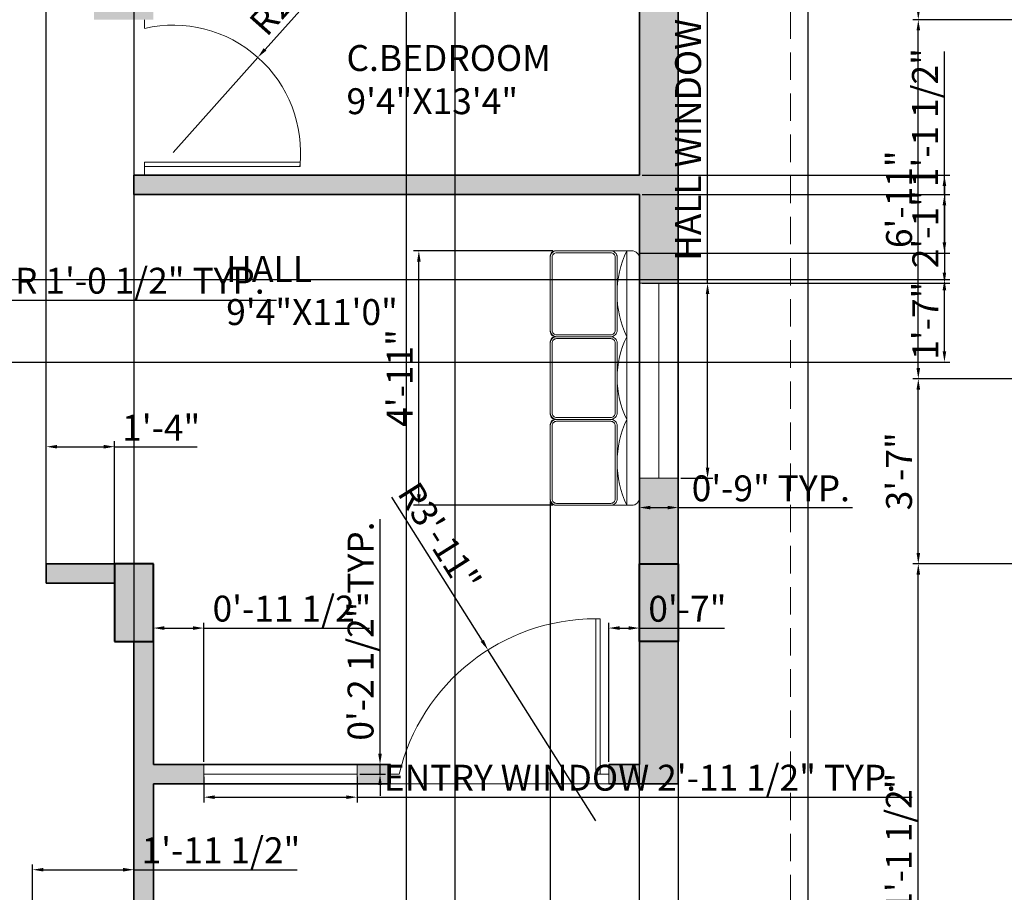
# Model space of a CAD drawing. Units: inches. Extents: x 2656 to 9931, y 1941 to 3068.
# Tile 3 of 46: x 2846 to 3074, y 2224 to 2426. Entities that reach past the tile are written whole.
import ezdxf

# ---------------------------------------------------------------- set-up
doc = ezdxf.new("R2010")
doc.units = ezdxf.units.IN
doc.linetypes.add('DASHED2', pattern=[9.525, 6.35, -3.175])
for name, color, linetype, lineweight in [('A-ANNO-DIMS', 2, 'Continuous', 18), ('A-AREA-IDEN', 7, 'Continuous', 18), ('A-COLS', 7, 'Continuous', 40), ('A-COLS-PATT', 146, 'Continuous', 13), ('A-DOOR', 3, 'Continuous', 18), ('A-FLOR-OVHD', 252, 'DASHED2', 13), ('A-FURN', 8, 'Continuous', 13), ('A-GLAZ', 4, 'Continuous', 18), ('A-WALL', 7, 'Continuous', 35), ('A-WALL-PATT', 251, 'Continuous', 13), ('C-PROP', 7, 'Continuous', 25)]:
    doc.layers.add(name, color=color, linetype=linetype, lineweight=lineweight)
doc.styles.get("Standard").update_dxf_attribs({"font": 'arial.ttf'})
doc.dimstyles.new('ISO-25', dxfattribs={"dimtxt": 6, "dimasz": 2.5, "dimexe": 1.25, "dimexo": 0.625, "dimtad": 1, "dimdec": 0, "dimlunit": 3, "dimtxsty": 'Standard', "dimcen": 2.5, "dimadec": 0, "dimazin": 0, "dimtfac": 1, "dimtdec": 0, "dimtmove": 0, "dimatfit": 3, "dimfxl": 1, "dimarcsym": 0})

# ---------------------------------------------------------------- blocks, each defined once
blk = doc.blocks.new('DOOR-BEDROOM-HALL')
for p, q in [((-0.04, 0), (-0.04, 36)), ((2.43, 36), (2.43, 34)), ((38.43, 3), (2.43, 3)), ((2.43, 3), (2.43, 2)), ((38.43, 2), (38.43, 3)), ((2.43, 0), (2.43, 2)), ((2.43, 2), (38.43, 2))]:
    blk.add_line(p, q)
blk.add_arc((9.01, 5.24), 29.5, 353.6889, 102.8962)
blk = doc.blocks.new('DOOR-ENTRY')
for p, q in [((48.56, 38.25), (47.56, 38.25)), ((47.56, 38.25), (47.56, 2.25)), ((48.56, 2.25), (48.56, 38.25)), ((0.04, 2.25), (2.04, 2.25)), ((0.04, 0), (50.56, 0)), ((47.56, 2.25), (48.56, 2.25)), ((50.56, 2.25), (48.56, 2.25))]:
    blk.add_line(p, q)
blk.add_arc((47.56, -8.52), 46.77, 90, 166.6828)
blk = doc.blocks.new('WIN-HALL')
for p, q in [((8.96, 45.14), (4.46, 45.14)), ((4.46, 45.14), (4.46, -0.02)), ((4.46, -0.02), (-0.04, -0.02))]:
    blk.add_line(p, q)
blk = doc.blocks.new('WIN-ENTRY')
for p, q in [((35.5, -0.05), (35.5, 2.2)), ((0.02, -0.05), (35.5, -0.05))]:
    blk.add_line(p, q)
blk = doc.blocks.new('*D47')
at = {"layer": 'A-ANNO-DIMS', "color": 0, "lineweight": -2, "transparency": 16777216}
for p, q in [((3004.93, 2365.04), (3004.93, 2467.44)), ((2998.78, 2365.04), (3006.18, 2365.04)), ((3004.93, 2322.38), (3004.93, 2362.54)), ((2998.78, 2319.88), (3006.18, 2319.88))]:
    blk.add_line(p, q, dxfattribs=at)
at = {"layer": 'A-ANNO-DIMS', "color": 0, "transparency": 16777216}
for points in [[(3004.51, 2362.54), (3005.35, 2362.54), (3004.93, 2365.04)], [(3004.51, 2322.38), (3005.35, 2322.38), (3004.93, 2319.88)]]:
    blk.add_solid(points, dxfattribs=at)
at = {"layer": 'Defpoints', "color": 0, "transparency": 16777216}
for p in [(2998.16, 2365.04), (3004.93, 2365.04), (2998.16, 2319.88)]:
    blk.add_point(p, dxfattribs=at)
at = {"layer": 'A-ANNO-DIMS', "color": 0, "transparency": 16777216, "insert": (3001.2, 2417.49), "char_height": 6, "attachment_point": 5, "rotation": 90}
blk.add_mtext('HALL WINDOW 3\'-9" TYP.', dxfattribs=at)
blk = doc.blocks.new('*D48')
at = {"layer": 'A-ANNO-DIMS', "color": 0, "lineweight": -2, "transparency": 16777216}
for p, q in [((2989.16, 2319.25), (2989.16, 2311.86)), ((2998.16, 2319.25), (2998.16, 2311.86)), ((2991.66, 2313.11), (2995.66, 2313.11)), ((2998.16, 2313.11), (3038.48, 2313.11))]:
    blk.add_line(p, q, dxfattribs=at)
at = {"layer": 'A-ANNO-DIMS', "color": 0, "transparency": 16777216}
for points in [[(2991.66, 2313.52), (2991.66, 2312.69), (2989.16, 2313.11)], [(2995.66, 2313.52), (2995.66, 2312.69), (2998.16, 2313.11)]]:
    blk.add_solid(points, dxfattribs=at)
at = {"layer": 'Defpoints', "color": 0, "transparency": 16777216}
for p in [(2989.16, 2319.88), (2998.16, 2319.88), (2998.16, 2313.11)]:
    blk.add_point(p, dxfattribs=at)
at = {"layer": 'A-ANNO-DIMS', "color": 0, "transparency": 16777216, "insert": (3019.57, 2316.79), "char_height": 6, "attachment_point": 5}
blk.add_mtext('0\'-9" TYP.', dxfattribs=at)
blk = doc.blocks.new('*D49')
at = {"layer": 'A-ANNO-DIMS', "color": 0, "lineweight": -2, "transparency": 16777216}
for p, q in [((2888.32, 2250.73), (2888.32, 2244.78)), ((2923.8, 2250.73), (2923.8, 2244.78)), ((2890.82, 2246.03), (2921.3, 2246.03)), ((2923.8, 2246.03), (3052.29, 2246.03))]:
    blk.add_line(p, q, dxfattribs=at)
at = {"layer": 'A-ANNO-DIMS', "color": 0, "transparency": 16777216}
for points in [[(2890.82, 2246.45), (2890.82, 2245.61), (2888.32, 2246.03)], [(2921.3, 2246.45), (2921.3, 2245.61), (2923.8, 2246.03)]]:
    blk.add_solid(points, dxfattribs=at)
at = {"layer": 'Defpoints', "color": 0, "transparency": 16777216}
for p in [(2888.32, 2251.35), (2923.8, 2251.35), (2923.8, 2246.03)]:
    blk.add_point(p, dxfattribs=at)
at = {"layer": 'A-ANNO-DIMS', "color": 0, "transparency": 16777216, "insert": (2989.29, 2249.76), "char_height": 6, "attachment_point": 5}
blk.add_mtext('ENTRY WINDOW 2\'-11 1/2" TYP.', dxfattribs=at)
blk = doc.blocks.new('*D50')
at = {"layer": 'A-ANNO-DIMS', "color": 0, "lineweight": -2, "transparency": 16777216}
for p, q in [((2929.12, 2256.1), (2929.12, 2310.4)), ((2924.42, 2253.6), (2930.37, 2253.6)), ((2929.12, 2251.35), (2929.12, 2253.6)), ((2924.42, 2251.35), (2930.37, 2251.35)), ((2929.12, 2248.85), (2929.12, 2246.35))]:
    blk.add_line(p, q, dxfattribs=at)
at = {"layer": 'A-ANNO-DIMS', "color": 0, "transparency": 16777216}
for points in [[(2928.7, 2256.1), (2929.53, 2256.1), (2929.12, 2253.6)], [(2928.7, 2248.85), (2929.53, 2248.85), (2929.12, 2251.35)]]:
    blk.add_solid(points, dxfattribs=at)
at = {"layer": 'Defpoints', "color": 0, "transparency": 16777216}
for p in [(2923.8, 2253.6), (2929.12, 2253.6), (2923.8, 2251.35)]:
    blk.add_point(p, dxfattribs=at)
at = {"layer": 'A-ANNO-DIMS', "color": 0, "transparency": 16777216, "insert": (2925.39, 2284.5), "char_height": 6, "attachment_point": 5, "rotation": 90}
blk.add_mtext('0\'-2 1/2" TYP.', dxfattribs=at)
blk = doc.blocks.new('*D61')
at = {"layer": 'A-ANNO-DIMS', "color": 0, "lineweight": -2, "transparency": 16777216}
for p, q in [((2778.76, 2362.36), (2778.76, 2359.89)), ((2781.26, 2361.14), (2788.58, 2361.14)), ((2791.08, 2362.36), (2791.08, 2359.89)), ((2791.08, 2361.14), (2905.16, 2361.14))]:
    blk.add_line(p, q, dxfattribs=at)
at = {"layer": 'A-ANNO-DIMS', "color": 0, "transparency": 16777216}
for points in [[(2781.26, 2361.55), (2781.26, 2360.72), (2778.76, 2361.14)], [(2788.58, 2361.55), (2788.58, 2360.72), (2791.08, 2361.14)]]:
    blk.add_solid(points, dxfattribs=at)
at = {"layer": 'Defpoints', "color": 0, "transparency": 16777216}
for p in [(2778.76, 2362.98), (2791.08, 2362.98), (2791.08, 2361.14)]:
    blk.add_point(p, dxfattribs=at)
at = {"layer": 'A-ANNO-DIMS', "color": 0, "transparency": 16777216, "insert": (2849.37, 2364.86), "char_height": 6, "attachment_point": 5}
blk.add_mtext('DINING CHAIR 1\'-0 1/2" TYP.', dxfattribs=at)
blk = doc.blocks.new('*D69')
at = {"layer": 'A-ANNO-DIMS', "color": 0, "lineweight": -2, "transparency": 16777216}
for p, q in [((3144.42, 2300.1), (3052.46, 2300.1)), ((3053.71, 2169.1), (3053.71, 2297.6)), ((3144.42, 2166.6), (3052.46, 2166.6))]:
    blk.add_line(p, q, dxfattribs=at)
at = {"layer": 'A-ANNO-DIMS', "color": 0, "transparency": 16777216}
for points in [[(3053.3, 2297.6), (3054.13, 2297.6), (3053.71, 2300.1)], [(3053.3, 2169.1), (3054.13, 2169.1), (3053.71, 2166.6)]]:
    blk.add_solid(points, dxfattribs=at)
at = {"layer": 'Defpoints', "color": 0, "transparency": 16777216}
for p in [(3053.71, 2300.1), (3145.05, 2300.1), (3145.05, 2166.6)]:
    blk.add_point(p, dxfattribs=at)
at = {"layer": 'A-ANNO-DIMS', "color": 0, "transparency": 16777216, "insert": (3049.99, 2233.35), "char_height": 6, "attachment_point": 5, "rotation": 90}
blk.add_mtext('11\'-1 1/2"', dxfattribs=at)
blk = doc.blocks.new('*D70')
at = {"layer": 'A-ANNO-DIMS', "color": 0, "lineweight": -2, "transparency": 16777216}
for p, q in [((3088.25, 2342.93), (3052.46, 2342.93)), ((3053.71, 2302.6), (3053.71, 2340.43)), ((3144.42, 2300.1), (3052.46, 2300.1))]:
    blk.add_line(p, q, dxfattribs=at)
at = {"layer": 'A-ANNO-DIMS', "color": 0, "transparency": 16777216}
for points in [[(3053.3, 2340.43), (3054.13, 2340.43), (3053.71, 2342.93)], [(3053.3, 2302.6), (3054.13, 2302.6), (3053.71, 2300.1)]]:
    blk.add_solid(points, dxfattribs=at)
at = {"layer": 'Defpoints', "color": 0, "transparency": 16777216}
for p in [(3053.71, 2342.93), (3088.87, 2342.93), (3145.05, 2300.1)]:
    blk.add_point(p, dxfattribs=at)
at = {"layer": 'A-ANNO-DIMS', "color": 0, "transparency": 16777216, "insert": (3050.02, 2321.51), "char_height": 6, "attachment_point": 5, "rotation": 90}
blk.add_mtext('3\'-7"', dxfattribs=at)
blk = doc.blocks.new('*D71')
at = {"layer": 'A-ANNO-DIMS', "color": 0, "lineweight": -2, "transparency": 16777216}
for p, q in [((3144.42, 2426.1), (3052.46, 2426.1)), ((3053.71, 2345.43), (3053.71, 2423.6)), ((3088.25, 2342.93), (3052.46, 2342.93))]:
    blk.add_line(p, q, dxfattribs=at)
at = {"layer": 'A-ANNO-DIMS', "color": 0, "transparency": 16777216}
for points in [[(3053.3, 2423.6), (3054.13, 2423.6), (3053.71, 2426.1)], [(3053.3, 2345.43), (3054.13, 2345.43), (3053.71, 2342.93)]]:
    blk.add_solid(points, dxfattribs=at)
at = {"layer": 'Defpoints', "color": 0, "transparency": 16777216}
for p in [(3053.71, 2426.1), (3145.05, 2426.1), (3088.87, 2342.93)]:
    blk.add_point(p, dxfattribs=at)
at = {"layer": 'A-ANNO-DIMS', "color": 0, "transparency": 16777216, "insert": (3050.03, 2384.51), "char_height": 6, "attachment_point": 5, "rotation": 90}
blk.add_mtext('6\'-11"', dxfattribs=at)
blk = doc.blocks.new('*D72')
at = {"layer": 'A-ANNO-DIMS', "color": 0, "lineweight": -2, "transparency": 16777216}
for p, q in [((3144.42, 2484.03), (3052.46, 2484.03)), ((3053.71, 2428.6), (3053.71, 2481.53)), ((3144.42, 2426.1), (3052.46, 2426.1))]:
    blk.add_line(p, q, dxfattribs=at)
at = {"layer": 'A-ANNO-DIMS', "color": 0, "transparency": 16777216}
for points in [[(3053.3, 2481.53), (3054.13, 2481.53), (3053.71, 2484.03)], [(3053.3, 2428.6), (3054.13, 2428.6), (3053.71, 2426.1)]]:
    blk.add_solid(points, dxfattribs=at)
at = {"layer": 'Defpoints', "color": 0, "transparency": 16777216}
for p in [(3053.71, 2484.03), (3145.05, 2484.03), (3145.05, 2426.1)]:
    blk.add_point(p, dxfattribs=at)
at = {"layer": 'A-ANNO-DIMS', "color": 0, "transparency": 16777216, "insert": (3050.03, 2455.07), "char_height": 6, "attachment_point": 5, "rotation": 90}
blk.add_mtext('4\'-10"', dxfattribs=at)
blk = doc.blocks.new('*D74')
at = {"layer": 'A-ANNO-DIMS', "color": 0, "lineweight": -2, "transparency": 16777216}
for p, q in [((2989.78, 2390.1), (3061.01, 2390.1)), ((3059.76, 2387.6), (3059.76, 2367.54)), ((2989.78, 2365.04), (3061.01, 2365.04))]:
    blk.add_line(p, q, dxfattribs=at)
at = {"layer": 'A-ANNO-DIMS', "color": 0, "transparency": 16777216}
for points in [[(3059.34, 2387.6), (3060.17, 2387.6), (3059.76, 2390.1)], [(3059.34, 2367.54), (3060.17, 2367.54), (3059.76, 2365.04)]]:
    blk.add_solid(points, dxfattribs=at)
at = {"layer": 'Defpoints', "color": 0, "transparency": 16777216}
for p in [(2989.16, 2390.1), (2989.16, 2365.04), (3059.76, 2365.04)]:
    blk.add_point(p, dxfattribs=at)
at = {"layer": 'A-ANNO-DIMS', "color": 0, "transparency": 16777216, "insert": (3056.12, 2377.57), "char_height": 6, "attachment_point": 5, "rotation": 90}
blk.add_mtext('2\'-1"', dxfattribs=at)
blk = doc.blocks.new('*D101')
at = {"layer": 'A-ANNO-DIMS', "color": 0, "lineweight": -2, "transparency": 16777216}
for p, q in [((2935.16, 2553.98), (2935.16, 2009.27)), ((2946.47, 2553.98), (2946.47, 2009.27)), ((2937.66, 2010.52), (2943.97, 2010.52)), ((2946.47, 2010.52), (2984.81, 2010.52))]:
    blk.add_line(p, q, dxfattribs=at)
at = {"layer": 'A-ANNO-DIMS', "color": 0, "transparency": 16777216}
for points in [[(2937.66, 2010.94), (2937.66, 2010.11), (2935.16, 2010.52)], [(2943.97, 2010.94), (2943.97, 2010.11), (2946.47, 2010.52)]]:
    blk.add_solid(points, dxfattribs=at)
at = {"layer": 'Defpoints', "color": 0, "transparency": 16777216}
for p in [(2935.16, 2554.6), (2946.47, 2554.6), (2946.47, 2010.52)]:
    blk.add_point(p, dxfattribs=at)
at = {"layer": 'A-ANNO-DIMS', "color": 0, "transparency": 16777216, "insert": (2966.89, 2014.25), "char_height": 6, "attachment_point": 5}
blk.add_mtext('0\'-11 1/2"', dxfattribs=at)
blk = doc.blocks.new('*D102')
at = {"layer": 'A-ANNO-DIMS', "color": 0, "lineweight": -2, "transparency": 16777216}
for p, q in [((2998.16, 2604.98), (2998.16, 2009.27)), ((2872.16, 2564.71), (2872.16, 2009.27)), ((2874.66, 2010.52), (2995.66, 2010.52))]:
    blk.add_line(p, q, dxfattribs=at)
at = {"layer": 'A-ANNO-DIMS', "color": 0, "transparency": 16777216}
for points in [[(2874.66, 2010.94), (2874.66, 2010.11), (2872.16, 2010.52)], [(2995.66, 2010.94), (2995.66, 2010.11), (2998.16, 2010.52)]]:
    blk.add_solid(points, dxfattribs=at)
at = {"layer": 'Defpoints', "color": 0, "transparency": 16777216}
for p in [(2998.16, 2605.6), (2872.16, 2565.34), (2998.16, 2010.52)]:
    blk.add_point(p, dxfattribs=at)
at = {"layer": 'A-ANNO-DIMS', "color": 0, "transparency": 16777216, "insert": (2935.16, 2014.21), "char_height": 6, "attachment_point": 5}
blk.add_mtext('10\'-6"', dxfattribs=at)
blk = doc.blocks.new('*D104')
at = {"layer": 'A-ANNO-DIMS', "color": 0, "lineweight": -2, "transparency": 16777216}
for p, q in [((2982.06, 2254.23), (2982.06, 2286.45)), ((2989.16, 2254.23), (2989.16, 2286.45)), ((2984.56, 2285.2), (2986.66, 2285.2)), ((2989.16, 2285.2), (3008.86, 2285.2))]:
    blk.add_line(p, q, dxfattribs=at)
at = {"layer": 'A-ANNO-DIMS', "color": 0, "transparency": 16777216}
for points in [[(2984.56, 2285.62), (2984.56, 2284.78), (2982.06, 2285.2)], [(2986.66, 2285.62), (2986.66, 2284.78), (2989.16, 2285.2)]]:
    blk.add_solid(points, dxfattribs=at)
at = {"layer": 'Defpoints', "color": 0, "transparency": 16777216}
for p in [(2989.16, 2285.2), (2982.06, 2253.6), (2989.16, 2253.6)]:
    blk.add_point(p, dxfattribs=at)
at = {"layer": 'A-ANNO-DIMS', "color": 0, "transparency": 16777216, "insert": (3000.26, 2288.89), "char_height": 6, "attachment_point": 5}
blk.add_mtext('0\'-7"', dxfattribs=at)
blk = doc.blocks.new('*D105')
at = {"layer": 'A-ANNO-DIMS', "color": 0, "lineweight": -2, "transparency": 16777216}
for p, q in [((2876.66, 2254.23), (2876.66, 2286.45)), ((2888.32, 2254.23), (2888.32, 2286.45)), ((2879.16, 2285.2), (2885.82, 2285.2)), ((2888.32, 2285.2), (2926.66, 2285.2))]:
    blk.add_line(p, q, dxfattribs=at)
at = {"layer": 'A-ANNO-DIMS', "color": 0, "transparency": 16777216}
for points in [[(2879.16, 2285.62), (2879.16, 2284.78), (2876.66, 2285.2)], [(2885.82, 2285.62), (2885.82, 2284.78), (2888.32, 2285.2)]]:
    blk.add_solid(points, dxfattribs=at)
at = {"layer": 'Defpoints', "color": 0, "transparency": 16777216}
for p in [(2888.32, 2285.2), (2876.66, 2253.6), (2888.32, 2253.6)]:
    blk.add_point(p, dxfattribs=at)
at = {"layer": 'A-ANNO-DIMS', "color": 0, "transparency": 16777216, "insert": (2908.74, 2288.93), "char_height": 6, "attachment_point": 5}
blk.add_mtext('0\'-11 1/2"', dxfattribs=at)
blk = doc.blocks.new('*D114')
at = {"layer": 'A-ANNO-DIMS', "color": 0, "lineweight": -2, "transparency": 16777216}
for p, q in [((2809.77, 2300.73), (2809.77, 2674.45)), ((2851.88, 2300.73), (2851.88, 2674.45)), ((2812.27, 2673.2), (2849.38, 2673.2))]:
    blk.add_line(p, q, dxfattribs=at)
at = {"layer": 'A-ANNO-DIMS', "color": 0, "transparency": 16777216}
for points in [[(2812.27, 2673.62), (2812.27, 2672.78), (2809.77, 2673.2)], [(2849.38, 2673.62), (2849.38, 2672.78), (2851.88, 2673.2)]]:
    blk.add_solid(points, dxfattribs=at)
at = {"layer": 'Defpoints', "color": 0, "transparency": 16777216}
for p in [(2851.88, 2673.2), (2809.77, 2300.1), (2851.88, 2300.1)]:
    blk.add_point(p, dxfattribs=at)
at = {"layer": 'A-ANNO-DIMS', "color": 0, "transparency": 16777216, "insert": (2830.82, 2676.89), "char_height": 6, "attachment_point": 5}
blk.add_mtext('3\'-6"', dxfattribs=at)
blk = doc.blocks.new('*D115')
at = {"layer": 'A-ANNO-DIMS', "color": 0, "lineweight": -2, "transparency": 16777216}
for p, q in [((2851.88, 2296.23), (2851.88, 2328.45)), ((2854.38, 2327.2), (2865.16, 2327.2)), ((2867.66, 2296.23), (2867.66, 2328.45)), ((2867.66, 2327.2), (2886.79, 2327.2))]:
    blk.add_line(p, q, dxfattribs=at)
at = {"layer": 'A-ANNO-DIMS', "color": 0, "transparency": 16777216}
for points in [[(2854.38, 2327.62), (2854.38, 2326.78), (2851.88, 2327.2)], [(2865.16, 2327.62), (2865.16, 2326.78), (2867.66, 2327.2)]]:
    blk.add_solid(points, dxfattribs=at)
at = {"layer": 'Defpoints', "color": 0, "transparency": 16777216}
for p in [(2867.66, 2327.2), (2851.88, 2295.6), (2867.66, 2295.6)]:
    blk.add_point(p, dxfattribs=at)
at = {"layer": 'A-ANNO-DIMS', "color": 0, "transparency": 16777216, "insert": (2878.47, 2330.84), "char_height": 6, "attachment_point": 5}
blk.add_mtext('1\'-4"', dxfattribs=at)
blk = doc.blocks.new('*D121')
at = {"layer": 'A-ANNO-DIMS', "color": 0, "lineweight": -2, "transparency": 16777216}
for p, q in [((2848.69, 2198.26), (2848.69, 2230.48)), ((2851.19, 2229.23), (2869.66, 2229.23)), ((2872.16, 2198.26), (2872.16, 2230.48)), ((2872.16, 2229.23), (2909.93, 2229.23))]:
    blk.add_line(p, q, dxfattribs=at)
at = {"layer": 'A-ANNO-DIMS', "color": 0, "transparency": 16777216}
for points in [[(2851.19, 2229.65), (2851.19, 2228.82), (2848.69, 2229.23)], [(2869.66, 2229.65), (2869.66, 2228.82), (2872.16, 2229.23)]]:
    blk.add_solid(points, dxfattribs=at)
at = {"layer": 'Defpoints', "color": 0, "transparency": 16777216}
for p in [(2872.16, 2229.23), (2848.69, 2197.63), (2872.16, 2197.63)]:
    blk.add_point(p, dxfattribs=at)
at = {"layer": 'A-ANNO-DIMS', "color": 0, "transparency": 16777216, "insert": (2892.3, 2232.96), "char_height": 6, "attachment_point": 5}
blk.add_mtext('1\'-11 1/2"', dxfattribs=at)
blk = doc.blocks.new('*D133')
at = {"layer": 'A-ANNO-DIMS', "color": 0, "lineweight": -2, "transparency": 16777216}
for p, q in [((2806.59, 2365.93), (3061.01, 2365.93)), ((3059.76, 2349.31), (3059.76, 2363.43)), ((2806.59, 2346.81), (3061.01, 2346.81))]:
    blk.add_line(p, q, dxfattribs=at)
at = {"layer": 'A-ANNO-DIMS', "color": 0, "transparency": 16777216}
for points in [[(3059.34, 2363.43), (3060.17, 2363.43), (3059.76, 2365.93)], [(3059.34, 2349.31), (3060.17, 2349.31), (3059.76, 2346.81)]]:
    blk.add_solid(points, dxfattribs=at)
at = {"layer": 'Defpoints', "color": 0, "transparency": 16777216}
for p in [(2805.96, 2365.93), (3059.76, 2365.93), (2805.96, 2346.81)]:
    blk.add_point(p, dxfattribs=at)
at = {"layer": 'A-ANNO-DIMS', "color": 0, "transparency": 16777216, "insert": (3056.12, 2356.37), "char_height": 6, "attachment_point": 5, "rotation": 90}
blk.add_mtext('1\'-7"', dxfattribs=at)
blk = doc.blocks.new('*D141')
at = {"layer": 'A-ANNO-DIMS', "color": 0, "lineweight": -2, "transparency": 16777216}
for p, q in [((2969.08, 2372.57), (2936.86, 2372.57)), ((2938.11, 2316.14), (2938.11, 2370.07)), ((2969.08, 2313.64), (2936.86, 2313.64))]:
    blk.add_line(p, q, dxfattribs=at)
at = {"layer": 'A-ANNO-DIMS', "color": 0, "transparency": 16777216}
for points in [[(2937.69, 2370.07), (2938.53, 2370.07), (2938.11, 2372.57)], [(2937.69, 2316.14), (2938.53, 2316.14), (2938.11, 2313.64)]]:
    blk.add_solid(points, dxfattribs=at)
at = {"layer": 'Defpoints', "color": 0, "transparency": 16777216}
for p in [(2938.11, 2372.57), (2969.71, 2372.57), (2969.71, 2313.64)]:
    blk.add_point(p, dxfattribs=at)
at = {"layer": 'A-ANNO-DIMS', "color": 0, "transparency": 16777216, "insert": (2934.47, 2343.11), "char_height": 6, "attachment_point": 5, "rotation": 90}
blk.add_mtext('4\'-11"', dxfattribs=at)
blk = doc.blocks.new('*D142')
at = {"layer": 'A-ANNO-DIMS', "color": 0, "lineweight": -2, "transparency": 16777216}
for p, q in [((2968.53, 2314.49), (2968.53, 2009.27)), ((2989.12, 2314.44), (2989.12, 2009.27)), ((2971.03, 2010.52), (2986.62, 2010.52)), ((2989.12, 2010.52), (3022.24, 2010.52))]:
    blk.add_line(p, q, dxfattribs=at)
at = {"layer": 'A-ANNO-DIMS', "color": 0, "transparency": 16777216}
for points in [[(2971.03, 2010.94), (2971.03, 2010.11), (2968.53, 2010.52)], [(2986.62, 2010.94), (2986.62, 2010.11), (2989.12, 2010.52)]]:
    blk.add_solid(points, dxfattribs=at)
at = {"layer": 'Defpoints', "color": 0, "transparency": 16777216}
for p in [(2968.53, 2315.11), (2989.12, 2315.06), (2989.12, 2010.52)]:
    blk.add_point(p, dxfattribs=at)
at = {"layer": 'A-ANNO-DIMS', "color": 0, "transparency": 16777216, "insert": (3006.93, 2014.25), "char_height": 6, "attachment_point": 5}
blk.add_mtext('1\'-8 1/2"', dxfattribs=at)
blk = doc.blocks.new('*D143')
at = {"layer": 'A-ANNO-DIMS', "color": 0, "lineweight": -2, "transparency": 16777216}
for p, q in [((3059.76, 2385.6), (3059.76, 2418.72)), ((2989.78, 2385.6), (3061.01, 2385.6)), ((3059.76, 2374.55), (3059.76, 2383.1)), ((2989.26, 2372.05), (3061.01, 2372.05))]:
    blk.add_line(p, q, dxfattribs=at)
at = {"layer": 'A-ANNO-DIMS', "color": 0, "transparency": 16777216}
for points in [[(3059.34, 2383.1), (3060.17, 2383.1), (3059.76, 2385.6)], [(3059.34, 2374.55), (3060.17, 2374.55), (3059.76, 2372.05)]]:
    blk.add_solid(points, dxfattribs=at)
at = {"layer": 'Defpoints', "color": 0, "transparency": 16777216}
for p in [(2989.16, 2385.6), (3059.76, 2385.6), (2988.64, 2372.05)]:
    blk.add_point(p, dxfattribs=at)
at = {"layer": 'A-ANNO-DIMS', "color": 0, "transparency": 16777216, "insert": (3056.03, 2403.41), "char_height": 6, "attachment_point": 5, "rotation": 90}
blk.add_mtext('1\'-1 1/2"', dxfattribs=at)
blk = doc.blocks.new('*D185')
at = {"layer": 'A-ANNO-DIMS', "color": 0, "lineweight": -2, "transparency": 16777216}
for p, q in [((2928.73, 2448.66), (2902.51, 2419.23)), ((2881.21, 2395.34), (2900.84, 2417.37))]:
    blk.add_line(p, q, dxfattribs=at)
at = {"layer": 'A-ANNO-DIMS', "color": 0, "transparency": 16777216}
blk.add_solid([(2902.19, 2419.51), (2902.82, 2418.96), (2900.84, 2417.37)], dxfattribs=at)
at = {"layer": 'Defpoints', "color": 0, "transparency": 16777216}
for p in [(2900.84, 2417.37), (2881.21, 2395.34)]:
    blk.add_point(p, dxfattribs=at)
at = {"layer": 'A-ANNO-DIMS', "color": 0, "transparency": 16777216, "insert": (2913.67, 2437.36), "char_height": 6, "attachment_point": 5, "rotation": 48.2926}
blk.add_mtext('R2\'-5 1/2"', dxfattribs=at)
blk = doc.blocks.new('*D188')
at = {"layer": 'A-ANNO-DIMS', "color": 0, "lineweight": -2, "transparency": 16777216}
for p, q in [((2931.78, 2315.55), (2952.78, 2282.26)), ((2979.06, 2240.58), (2954.11, 2280.14))]:
    blk.add_line(p, q, dxfattribs=at)
at = {"layer": 'A-ANNO-DIMS', "color": 0, "transparency": 16777216}
blk.add_solid([(2953.13, 2282.48), (2952.42, 2282.03), (2954.11, 2280.14)], dxfattribs=at)
at = {"layer": 'Defpoints', "color": 0, "transparency": 16777216}
for p in [(2954.11, 2280.14), (2979.06, 2240.58)]:
    blk.add_point(p, dxfattribs=at)
at = {"layer": 'A-ANNO-DIMS', "color": 0, "transparency": 16777216, "insert": (2942.26, 2305.85), "char_height": 6, "attachment_point": 5, "rotation": 302.235}
blk.add_mtext('R3\'-11"', dxfattribs=at)

msp = doc.modelspace()

# ---------------------------------------------------------------- hatches: boundary and pattern name
at = {"layer": 'A-COLS-PATT'}
h = msp.add_hatch(color=256, dxfattribs=at)
h.dxf.hatch_style = 1
h.paths.add_polyline_path([(2752.16, 2623.6), (2743.16, 2623.6), (2743.16, 2605.6), (2752.16, 2605.6)])
h.paths.add_polyline_path([(2876.66, 2623.6), (2858.66, 2623.6), (2858.66, 2614.6), (2876.66, 2614.6)])
h.paths.add_polyline_path([(2998.16, 2623.6), (2989.16, 2623.6), (2989.16, 2614.6), (2989.16, 2605.6), (2998.16, 2605.6)])
h.paths.add_polyline_path([(2998.16, 2444.1), (2989.16, 2444.1), (2989.16, 2426.1), (2998.16, 2426.1)])
h.paths.add_polyline_path([(2876.66, 2444.1), (2867.66, 2444.1), (2867.66, 2426.1), (2876.66, 2426.1)])
h.paths.add_polyline_path([(2752.16, 2444.1), (2743.16, 2444.1), (2743.16, 2426.1), (2752.16, 2426.1)])
h.paths.add_polyline_path([(2752.16, 2300.1), (2743.16, 2300.1), (2743.16, 2282.1), (2752.16, 2282.1)])
h.paths.add_polyline_path([(2876.66, 2300.1), (2867.66, 2300.1), (2867.66, 2282.1), (2876.66, 2282.1)])
h.paths.add_polyline_path([(2998.16, 2300.1), (2989.16, 2300.1), (2989.16, 2282.1), (2998.16, 2282.1)])
h.paths.add_polyline_path([(2998.16, 2184.6), (2989.16, 2184.6), (2989.16, 2166.6), (2998.16, 2166.6)])
h.paths.add_polyline_path([(2876.66, 2175.6), (2858.66, 2175.6), (2858.66, 2166.6), (2876.66, 2166.6)])
h.paths.add_polyline_path([(2752.16, 2184.6), (2743.16, 2184.6), (2743.16, 2166.6), (2752.16, 2166.6)])
at = {"layer": 'A-WALL-PATT'}
h = msp.add_hatch(color=256, dxfattribs=at)
h.dxf.hatch_style = 1
h.paths.add_polyline_path([(2858.66, 2623.6), (2752.16, 2623.6), (2752.16, 2614.6), (2858.66, 2614.6)])
h.paths.add_polyline_path([(2893.09, 2623.6), (2876.66, 2623.6), (2876.66, 2614.6), (2893.09, 2614.6), (2893.09, 2619.1)])
h.paths.add_polyline_path([(2946.51, 2623.6), (2917.09, 2623.6), (2917.09, 2614.6), (2946.51, 2614.6), (2946.51, 2619.1)])
h.paths.add_polyline_path([(2989.16, 2623.6), (2970.51, 2623.6), (2970.51, 2614.6), (2989.16, 2614.6)])
h.paths.add_polyline_path([(2998.16, 2605.6), (2989.16, 2605.6), (2989.16, 2523.88), (2998.16, 2523.88)])
h.paths.add_polyline_path([(2935.16, 2614.6), (2930.66, 2614.6), (2930.66, 2554.6), (2876.66, 2554.6), (2876.66, 2565.34), (2872.16, 2565.34), (2872.16, 2444.1), (2876.66, 2444.1), (2876.66, 2550.1), (2946.47, 2550.1), (2946.47, 2554.6), (2935.16, 2554.6)])
h.paths.add_polyline_path([(2989.16, 2554.6), (2982.11, 2554.6), (2976.57, 2554.6), (2976.57, 2550.1), (2982.11, 2550.1), (2989.16, 2550.1)])
h.paths.add_polyline_path([(2876.66, 2614.6), (2872.16, 2614.6), (2872.16, 2595), (2876.66, 2595)], flags=0)
h.paths.add_polyline_path([(2752.16, 2605.6), (2743.16, 2605.6), (2743.16, 2544.03), (2752.16, 2544.03)])
h.paths.add_polyline_path([(2752.16, 2426.1), (2743.16, 2426.1), (2743.16, 2300.1), (2752.16, 2300.1)])
h.paths.add_polyline_path([(2821.13, 2430.6), (2752.16, 2430.6), (2752.16, 2426.1), (2821.13, 2426.1)])
h.paths.add_polyline_path([(2867.66, 2430.6), (2862.88, 2430.6), (2862.88, 2426.1), (2867.66, 2426.1)])
h.paths.add_polyline_path([(2752.16, 2484.03), (2747.66, 2484.03), (2743.16, 2484.03), (2743.16, 2444.1), (2752.16, 2444.1)])
h.paths.add_polyline_path([(2998.16, 2426.1), (2989.16, 2426.1), (2989.16, 2390.1), (2872.16, 2390.1), (2872.16, 2385.6), (2876.66, 2385.6), (2989.16, 2385.6), (2989.16, 2365.04), (2998.16, 2365.04)])
h.paths.add_polyline_path([(2998.16, 2463.88), (2993.66, 2463.88), (2989.16, 2463.88), (2989.16, 2444.1), (2998.16, 2444.1)])
h.paths.add_polyline_path([(2998.16, 2319.88), (2989.16, 2319.88), (2989.16, 2300.1), (2998.16, 2300.1)])
h.paths.add_polyline_path([(2998.16, 2282.1), (2989.16, 2282.1), (2989.16, 2253.6), (2982.06, 2253.6), (2982.06, 2249.1), (2989.16, 2249.1), (2998.16, 2249.1)])
h.paths.add_polyline_path([(2931.54, 2253.6), (2923.8, 2253.6), (2923.8, 2249.1), (2931.54, 2249.1)])
h.paths.add_polyline_path([(2876.66, 2282.1), (2872.16, 2282.1), (2872.16, 2184.6), (2872.16, 2175.6), (2876.66, 2175.6), (2876.66, 2249.1), (2888.32, 2249.1), (2888.32, 2251.35), (2888.32, 2253.6), (2876.66, 2253.6)])
h.paths.add_polyline_path([(2858.66, 2175.6), (2841.42, 2175.6), (2841.42, 2166.6), (2858.66, 2166.6)])
h.paths.add_polyline_path([(2785.06, 2171.1), (2785.06, 2175.6), (2752.16, 2175.6), (2752.16, 2166.6), (2785.06, 2166.6)])
h.paths.add_polyline_path([(2752.16, 2282.1), (2743.16, 2282.1), (2743.16, 2184.6), (2752.16, 2184.6)])
h.paths.add_polyline_path([(2809.77, 2300.1), (2752.16, 2300.1), (2752.16, 2295.6), (2809.77, 2295.6)])
h.paths.add_polyline_path([(2867.66, 2300.1), (2851.88, 2300.1), (2851.88, 2295.6), (2867.66, 2295.6)])

# ---------------------------------------------------------------- linework, layer by layer
at = {"layer": 'A-COLS'}
for p, q in [((2876.66, 2300.1), (2867.66, 2300.1)), ((2867.66, 2300.1), (2867.66, 2282.1)), ((2876.66, 2282.1), (2876.66, 2300.1)), ((2989.16, 2300.1), (2998.16, 2300.1)), ((2989.16, 2282.1), (2989.16, 2300.1)), ((2998.16, 2300.1), (2998.16, 2282.1)), ((2867.66, 2282.1), (2876.66, 2282.1)), ((2998.16, 2282.1), (2989.16, 2282.1)), ((2989.16, 2282.1), (2989.16, 2282.1))]:
    msp.add_line(p, q, dxfattribs=at)
at = {"layer": 'A-DOOR'}
for p, q in [((2931.54, 2253.6), (2931.54, 2249.1)), ((2982.06, 2253.6), (2982.06, 2249.1))]:
    msp.add_line(p, q, dxfattribs=at)
at = {"layer": 'A-FLOR-OVHD'}
msp.add_line((3024.16, 2637.6), (3024.16, 2090.1), dxfattribs=at)
at = {"layer": 'A-FURN'}
for points in [[(2970, 2352.68), (2982.53, 2352.68, 0.414214), (2984, 2354.16), (2984, 2371.1, 0.414214), (2982.53, 2372.57), (2970, 2372.57, 0.414214), (2968.53, 2371.1), (2968.53, 2354.16, 0.414214)], [(2970, 2353.12), (2982.53, 2353.12, 0.414214), (2983.56, 2354.16), (2983.56, 2371.1, 0.414214), (2982.53, 2372.13), (2970, 2372.13, 0.414214), (2968.97, 2371.1), (2968.97, 2354.16, 0.414214)], [(2970, 2352.68), (2982.53, 2352.68, -0.414214), (2984, 2351.21), (2984, 2335, -0.414214), (2982.53, 2333.53), (2970, 2333.53, -0.414214), (2968.53, 2335), (2968.53, 2351.21, -0.414214)], [(2970, 2352.24), (2982.53, 2352.24, -0.414214), (2983.56, 2351.21), (2983.56, 2335, -0.414214), (2982.53, 2333.97), (2970, 2333.97, -0.414214), (2968.97, 2335), (2968.97, 2351.21, -0.414214)], [(2970, 2313.64), (2982.53, 2313.64, 0.414214), (2984, 2315.11), (2984, 2332.06, 0.414214), (2982.53, 2333.53), (2970, 2333.53, 0.414214), (2968.53, 2332.06), (2968.53, 2315.11, 0.414214)], [(2970, 2314.08), (2982.53, 2314.08, 0.414214), (2983.56, 2315.11), (2983.56, 2332.06, 0.414214), (2982.53, 2333.09), (2970, 2333.09, 0.414214), (2968.97, 2332.06), (2968.97, 2315.11, 0.414214)]]:
    msp.add_lwpolyline(points, format="xyb", close=True, dxfattribs=at)
at = {"layer": 'A-FURN', "ltscale": 0.03}
msp.add_lwpolyline([(2968.53, 2332.34), (2968.53, 2314.82, 0.414214), (2969.71, 2313.64), (2987.39, 2313.64, 0.414214), (2989.16, 2315.41), (2989.16, 2370.8, 0.414214), (2987.39, 2372.57), (2969.71, 2372.57, 0.414214), (2968.53, 2371.39), (2968.53, 2353.88, 0.414214), (2969.71, 2352.7, -1), (2969.71, 2352.67, 0.414214), (2968.53, 2351.49), (2968.53, 2334.72, 0.414214), (2969.71, 2333.54, -1), (2969.71, 2333.52, 0.414214)], format="xyb", close=True, dxfattribs=at)
at = {"layer": 'A-FURN'}
msp.add_lwpolyline([(2986.21, 2313.64), (2986.21, 2372.57)], dxfattribs=at)
for centre, radius, start, end in [((3007.21, 2362.63), 23.23, 154.6538, 205.3462), ((3005.73, 2343.11), 21.74, 153.869, 206.131), ((3007.45, 2323.58), 23.45, 154.9106, 205.0894)]:
    msp.add_arc(centre, radius, start, end, dxfattribs=at)
at = {"layer": 'A-GLAZ'}
for p, q in [((2989.16, 2365.04), (2998.16, 2365.04)), ((2989.16, 2319.88), (2998.16, 2319.88)), ((2888.32, 2253.6), (2888.32, 2249.1)), ((2923.8, 2253.6), (2923.8, 2249.1)), ((2888.32, 2249.1), (2888.32, 2251.35))]:
    msp.add_line(p, q, dxfattribs=at)
at = {"layer": 'A-WALL'}
for p, q in [((2998.16, 2623.6), (2998.16, 2249.1)), ((2989.16, 2614.6), (2989.16, 2390.1)), ((2872.16, 2390.1), (2989.16, 2390.1)), ((2872.16, 2390.1), (2872.16, 2385.6)), ((2876.66, 2385.6), (2872.16, 2385.6)), ((2876.66, 2385.6), (2989.16, 2385.6)), ((2989.16, 2385.6), (2989.16, 2253.6)), ((2851.88, 2300.1), (2876.66, 2300.1)), ((2851.88, 2300.1), (2851.88, 2295.6)), ((2876.66, 2300.1), (2876.66, 2253.6)), ((2851.88, 2295.6), (2867.66, 2295.6)), ((2872.16, 2282.1), (2872.16, 2184.6)), ((2876.66, 2253.6), (2931.54, 2253.6)), ((2982.06, 2253.6), (2989.16, 2253.6)), ((2876.66, 2249.1), (2876.66, 2166.6)), ((2876.66, 2249.1), (2931.54, 2249.1)), ((2982.06, 2249.1), (2989.16, 2249.1)), ((2989.16, 2249.1), (2998.16, 2249.1))]:
    msp.add_line(p, q, dxfattribs=at)
at = {"layer": 'C-PROP'}
msp.add_line((3028.16, 2641.6), (3028.16, 2086.1), dxfattribs=at)

# ---------------------------------------------------------------- block references
at = {"layer": 'A-DOOR'}
for name, p in [('DOOR-BEDROOM-HALL', (2872.2, 2390.1)), ('DOOR-ENTRY', (2931.5, 2249.1))]:
    msp.add_blockref(name, p, dxfattribs=at)
at = {"layer": 'A-GLAZ'}
for name, p in [('WIN-HALL', (2989.2, 2319.9)), ('WIN-ENTRY', (2888.3, 2251.4))]:
    msp.add_blockref(name, p, dxfattribs=at)

# ---------------------------------------------------------------- texts
at = {"layer": 'A-AREA-IDEN', "char_height": 6, "attachment_point": 1}
for s, insert in [('C.BEDROOM\\P9\'4"X13\'4"', (2921.36, 2420.22)), ('HALL\\P9\'4"X11\'0"', (2893.52, 2371.38))]:
    msp.add_mtext_dynamic_manual_height_columns(s, width=137.4726, gutter_width=12.5, heights=[0], dxfattribs=dict(at, insert=insert))

# ---------------------------------------------------------------- dimensions: what is measured, and where the dimension line sits
at = {"layer": 'A-ANNO-DIMS'}
for base, p1, p2, picture, middle in [((2851.88, 2673.2), (2809.77, 2300.1), (2851.88, 2300.1), '*D114', (2830.82, 2676.89)), ((2998.16, 2010.52), (2872.16, 2565.34), (2998.16, 2605.6), '*D102', (2935.16, 2014.21)), ((2946.47, 2010.52), (2935.16, 2554.6), (2946.47, 2554.6), '*D101', (2966.89, 2014.25)), ((2867.66, 2327.2), (2851.88, 2295.6), (2867.66, 2295.6), '*D115', (2878.47, 2330.84)), ((2989.12, 2010.52), (2968.53, 2315.11), (2989.12, 2315.06), '*D142', (3006.93, 2014.25)), ((2888.32, 2285.2), (2876.66, 2253.6), (2888.32, 2253.6), '*D105', (2908.74, 2288.93)), ((2989.16, 2285.2), (2982.06, 2253.6), (2989.16, 2253.6), '*D104', (3000.26, 2288.89)), ((2872.16, 2229.23), (2848.69, 2197.63), (2872.16, 2197.63), '*D121', (2892.3, 2232.96))]:
    dim = msp.add_linear_dim(base=base, p1=p1, p2=p2, dimstyle='ISO-25', override={"dimdec": 1, "dimlfac": 1, "dimrnd": 0, "dimzin": 1, "dimdsep": 46, "dimlunit": 4, "dimfrac": 2}, dxfattribs=at)
    dim.commit()
    dim.dimension.update_dxf_attribs({"geometry": picture, "text_midpoint": middle})
for base, p1, p2, picture, middle in [((3053.71, 2484.03), (3145.05, 2426.1), (3145.05, 2484.03), '*D72', (3050.03, 2455.07)), ((3053.71, 2426.1), (3088.87, 2342.93), (3145.05, 2426.1), '*D71', (3050.03, 2384.51)), ((3059.7573, 2385.6003), (2988.6394, 2372.0545), (2989.1573, 2385.6003), '*D143', (3056.0299, 2403.4081)), ((3059.76, 2365.04), (2989.16, 2390.1), (2989.16, 2365.04), '*D74', (3056.12, 2377.57)), ((2938.11, 2372.57), (2969.71, 2313.64), (2969.71, 2372.57), '*D141', (2934.47, 2343.11)), ((3059.76, 2365.93), (2805.96, 2346.81), (2805.96, 2365.93), '*D133', (3056.12, 2356.37)), ((3053.71, 2342.93), (3145.05, 2300.1), (3088.87, 2342.93), '*D70', (3050.02, 2321.51)), ((3053.71, 2300.1), (3145.05, 2166.6), (3145.05, 2300.1), '*D69', (3049.99, 2233.35))]:
    dim = msp.add_linear_dim(base=base, p1=p1, p2=p2, angle=90, dimstyle='ISO-25', override={"dimdec": 1, "dimlfac": 1, "dimrnd": 0, "dimzin": 1, "dimdsep": 46, "dimlunit": 4, "dimfrac": 2}, dxfattribs=at)
    dim.commit()
    dim.dimension.update_dxf_attribs({"geometry": picture, "text_midpoint": middle})
for base, p1, p2, text, picture, middle in [((3004.93, 2365.04), (2998.16, 2319.88), (2998.16, 2365.04), 'HALL WINDOW <> TYP.', '*D47', (3001.2, 2417.49)), ((2929.116882, 2253.60027301), (2923.79588313, 2251.35027301), (2923.79588313, 2253.60027301), '<> TYP.', '*D50', (2925.38956276, 2284.50221708))]:
    dim = msp.add_linear_dim(base=base, p1=p1, p2=p2, angle=90, text=text, dimstyle='ISO-25', override={"dimdec": 1, "dimlfac": 1, "dimrnd": 0, "dimzin": 1, "dimdsep": 46, "dimlunit": 4, "dimfrac": 2}, dxfattribs=at)
    dim.commit()
    dim.dimension.update_dxf_attribs({"geometry": picture, "text_midpoint": middle})
dim = msp.add_radius_dim(center=(2881.21, 2395.34), mpoint=(2900.84, 2417.37), dimstyle='ISO-25', override={"dimdec": 1, "dimlfac": 1, "dimrnd": 0, "dimzin": 1, "dimdsep": 46, "dimlunit": 4, "dimfrac": 2}, dxfattribs=at)
dim.commit()
dim.dimension.update_dxf_attribs({"geometry": '*D185', "text_midpoint": (2913.67, 2437.36)})
for base, p1, p2, text, picture, middle in [((2791.08, 2361.14), (2778.76, 2362.98), (2791.08, 2362.98), 'DINING CHAIR <> TYP.', '*D61', (2849.37, 2364.86)), ((2998.16, 2313.11), (2989.16, 2319.88), (2998.16, 2319.88), '<> TYP.', '*D48', (3019.57, 2316.79)), ((2923.8, 2246.03), (2888.32, 2251.35), (2923.8, 2251.35), 'ENTRY WINDOW <> TYP.', '*D49', (2989.29, 2249.76))]:
    dim = msp.add_linear_dim(base=base, p1=p1, p2=p2, text=text, dimstyle='ISO-25', override={"dimdec": 1, "dimlfac": 1, "dimrnd": 0, "dimzin": 1, "dimdsep": 46, "dimlunit": 4, "dimfrac": 2}, dxfattribs=at)
    dim.commit()
    dim.dimension.update_dxf_attribs({"geometry": picture, "text_midpoint": middle})
dim = msp.add_radius_dim(center=(2979.06, 2240.58), mpoint=(2954.11, 2280.14), dimstyle='ISO-25', override={"dimdec": 1, "dimlfac": 1, "dimrnd": 0, "dimzin": 1, "dimdsep": 46, "dimlunit": 4, "dimfrac": 2}, dxfattribs=at)
dim.commit()
dim.dimension.update_dxf_attribs({"geometry": '*D188', "text_midpoint": (2939.14, 2303.88), "dimtype": 164})

doc.saveas('drawing.dxf')
